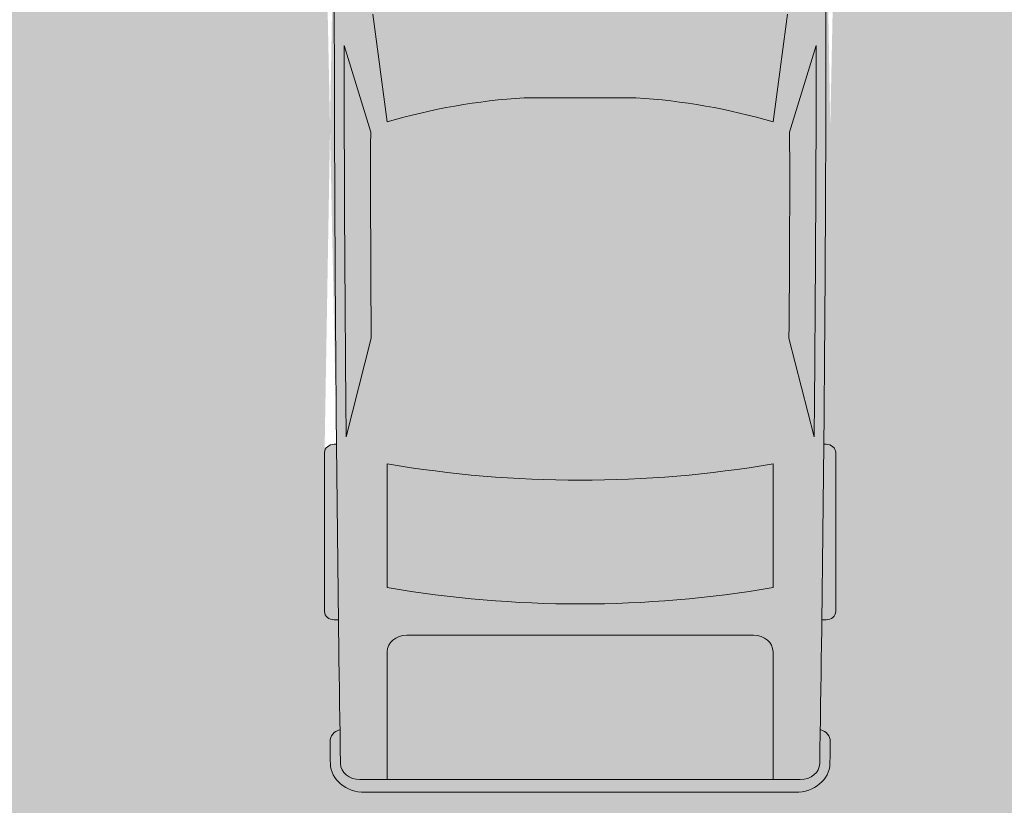
# Model space of a CAD drawing. Units: inches. Extents: x 389 to 971, y 148 to 870.
# Tile 1 of 14: x 448 to 565, y 256 to 349. Entities that reach past the tile are written whole.
import ezdxf

# ---------------------------------------------------------------- set-up
doc = ezdxf.new("R2010")
doc.units = ezdxf.units.IN
doc.header["$MEASUREMENT"] = 0
doc.layers.add('C-VEHI', color=8, linetype='Continuous', lineweight=13)
doc.layers.add('L-GRND-BASE-PATT', color=8, linetype='Continuous', lineweight=13)
doc.layers.add('C-VEHI-PATT', color=18, linetype='Continuous', lineweight=13, true_color=0x000000)
doc.layers.add('L-GRND-PATT', color=39, linetype='Continuous', lineweight=13, true_color=0x603913)

# ---------------------------------------------------------------- blocks, each defined once
blk = doc.blocks.new('*U7')
for p, q in [((136.6978032355602, 38.88847654282876), (160.90094244002, 38.88847654282867)), ((135.4513231603356, 37.07354110333037), (135.4513231603356, 37.40863046792069)), ((162.1474225152445, 37.40863046792049), (162.1474225152445, 36.77402019194128)), ((87.98532186932616, 31.87120872459877), (74.75900729854769, 35.92175679182955)), ((134.313356548143, 35.6043097713567), (119.2882629232503, 31.77757799177584)), ((186.4728846989705, -33.49860931502491), (186.4728846989718, 33.49860931502465)), ((70.0302824853563, 31.53613089391356), (86.40615155322342, 29.35124891408057)), ((188.3990091454065, -32.75868627757393), (188.3990091454077, 32.75868627757058)), ((138.4228833961707, 29.35124891408074), (157.2465674415997, 29.35124891408074)), ((186.4728846989718, 29.35124891408083), (167.0083537481071, 29.35124891408083)), ((164.515393597658, 26.39155676426461), (164.5153935976578, -26.39155676426503)), ((186.4728846989718, -10.5288681329018), (186.4728846989718, 10.52886813290129)), ((82.73706193978568, 8.496039918672748), (82.73706193978568, -8.49603991867258)), ((86.40615155322318, -29.35124891408145), (70.03028248535594, -31.53613089391442)), ((157.2465674415997, -29.35124891408117), (138.4228833961707, -29.35124891408126)), ((167.008353748107, -29.35124891408126), (186.4728846989707, -29.35124891408108)), ((87.98532186932607, -31.87120872459903), (74.7590072985476, -35.92175679182964)), ((134.3133565481428, -35.60430977135721), (119.2882629232503, -31.77757799177618)), ((135.4513231603355, -37.07354110333088), (135.4513231603355, -37.4086304679212)), ((162.1474225152445, -37.408630467921), (162.1474225152445, -36.77402019194179)), ((136.6978032355602, -38.88847654282927), (160.9009424400199, -38.88847654282918))]:
    blk.add_line(p, q)
for centre, major_axis, ratio, start_param, end_param in [((64.48199294511879, -10555.61767587835), (1.907644e-10, 10593.02630634627), 0.842303869543847, -0.0133969486112073, 0.0027970409639888), ((136.6978032355602, 37.40863046792072), (2.357e-13, -1.479846074908118), 0.842303869543976, 3.141592653589603, 4.712388980384554), ((160.90094244002, 37.40863046792052), (5.59e-14, 1.479846074908118), 0.842303869543976, -1.570796326794865, 4.44e-14), ((180.6280394947615, 35.8381667808375), (7.4e-14, 2.219769112362114), 0.8423038695439693, -0.0130174256259048, 1.249894140392862), ((64.48199294754608, -10556.35759891604), (1.349839377e-06, 10595.3130398087), 0.8423038681351469, -0.0133969484821159, -0.0130174254969711), ((183.9799245485216, 32.75868627756583), (8.56e-14, -5.246425615115243), 0.8423038695439737, 1.570796326795794, 3.128195704978164), ((183.9799245485226, 33.49860931502124), (3e-16, -2.959692149816168), 0.8423038695439952, 1.570796326796048, 3.128195704978389), ((64.4819929449925, -10555.61767590795), (1.9177683e-09, -10591.54646030096), 0.8423038695482963, 3.133765086725325, 3.140440689641252), ((95.78879860270445, -3666.353346297651), (1.949864e-10, -3698.236159209632), 0.8423038695446962, 3.134048706297306, 3.14409775411291), ((149.595361812917, 2.799442537139299), (8.561e-13, -79.57966406425402), 0.842303869543983, 4.372215489277867, 4.640744122441986), ((17.08207736189386, -1.421e-13), (6.87e-14, 147.0179238898305), 0.8423038695439764, 4.511394369635731, 4.913383591133647), ((35.90576140732288, -1.421e-13), (6.87e-14, 147.0179238898305), 0.8423038695439764, 4.511394369635731, 4.913383591133647), ((167.0083537481071, 26.39155676426464), (1.394e-13, 2.959692149816236), 0.842303869543976, 5.55e-14, 1.57079632679492), ((149.5953618129329, -2.799442537137565), (4.0897e-12, -79.57966406427697), 0.8423038695439419, -1.499151468852248, -1.230622835688196), ((167.008353748107, -26.39155676426503), (1.02e-14, -2.959692149816192), 0.8423038695439885, 4.712388980384686, 6.283185307179581), ((95.78879860271888, 3666.35334629765), (1.637818e-10, -3698.236159209629), 0.8423038695447546, -0.0025051005232382, 0.007543947292366), ((183.9799245485177, -32.7586862775633), (2.428e-13, -5.246425615118353), 0.8423038695439808, 0.0133969486110846, 1.570796326792831), ((183.9799245485216, -33.4986093150211), (9.3e-15, 2.959692149816141), 0.8423038695439732, 3.154989602201626, 4.71238898038339), ((64.48199294503607, 10555.61767590793), (1.6049794e-09, -10591.54646030094), 0.8423038695397146, 0.0011519639481523, 0.0078275668641468), ((64.48199294495228, 10555.61767590795), (6.117947e-10, 10593.02630637587), 0.8423038695458146, 3.138795612625926, 3.154989602201039), ((136.6978032355602, -37.40863046792109), (1.56e-14, -1.479846074908162), 0.8423038695440105, -1.570796326794875, -1.27e-14), ((160.9009424400199, -37.408630467921), (1.969e-13, 1.479846074908162), 0.8423038695440109, 3.141592653589951, 4.712388980384771), ((180.6280394947581, -35.83816678083949), (2.274e-13, -2.219769112363032), 0.8423038695439803, -1.249894138785958, 0.0130174256254374), ((64.48199294197605, 10556.3575989598), (9.365289701e-07, 10595.31303985772), 0.8423038705260315, 3.154610079306566, 3.154989602290631)]:
    blk.add_ellipse(centre, major_axis=major_axis, ratio=ratio, start_param=start_param, end_param=end_param)

msp = doc.modelspace()

# ---------------------------------------------------------------- hatches: boundary and pattern name
at = {"layer": 'C-VEHI-PATT'}
h = msp.add_hatch(color=256, dxfattribs=at)
h.dxf.hatch_style = 1
edge = h.paths.add_edge_path(flags=16)
edge.add_ellipse((3386.011413077446, 329.726312794031), major_axis=(-2896.629999631248, 1.069454e-10), ratio=0.8423038695494893, start_angle=-0.1208973690315247, end_angle=0.3640763488915013, ccw=False)
edge.add_line((489.3905023836935, 335.8383575186984), (486.2179253655185, 346.1978202249628))
edge.add_ellipse((8782.002602781096, 354.247254279773), major_axis=(-8295.790181758603, 9.87839e-10), ratio=0.8423038695486498, start_angle=0.0555943135052214, end_angle=0.3777641939157137)
edge.add_line((486.4665645878948, 299.5520931219791), (489.4638383140943, 311.3204429697198))
edge = h.paths.add_edge_path(flags=16)
edge.add_ellipse((512.1608573463288, 287.5825181681774), major_axis=(62.33048198263887, 2.0798e-12), ratio=0.8423038695439498, start_angle=94.8700695971331, end_angle=112.791914877584)
edge.add_line((491.3642517254777, 337.0752369161335), (489.6529508739416, 349.9015767089268))
edge.add_ellipse((510.1338164488795, 298.7862183048575), major_axis=(64.04807894948699, 3.9006e-12), ratio=0.8423038695439252, start_angle=94.27742096304979, end_angle=111.83495379670401, ccw=False)
edge.add_line((506.1068129054811, 352.6274231954524), (522.600208125781, 352.6274231954521))
edge.add_ellipse((518.5732045823798, 298.7862183048586), major_axis=(64.04807894948067, 3.24e-14), ratio=0.8423038695439885, start_angle=68.16504620328948, end_angle=85.72257903694378, ccw=False)
edge.add_line((539.05407015732, 349.9015767089259), (537.3427693057835, 337.0752369161327))
edge.add_ellipse((516.5461636849332, 287.5825181681899), major_axis=(62.33048198262021, 1.5954e-12), ratio=0.8423038695439995, start_angle=67.20808512240782, end_angle=85.12993040286212)
edge.add_line((521.0080028322477, 339.9490379899644), (507.6990181990146, 339.9490379899646))
edge = h.paths.add_edge_path(flags=16)
edge.add_ellipse((514.3535105156315, 391.3730654902235), major_axis=(-115.1512533244504, 1.8736e-12), ratio=0.8423038695439684, start_angle=76.4018653097696, end_angle=103.5981346902308)
edge.add_line((537.3427693057832, 296.3333211885938), (537.342769305783, 281.5897392316151))
edge.add_ellipse((514.3535105156313, 376.6294835332447), major_axis=(-115.1512533244486, 9.02e-13), ratio=0.8423038695439828, start_angle=76.40186530976922, end_angle=103.59813469023032, ccw=False)
edge.add_line((491.3642517254773, 281.5897392316156), (491.3642517254774, 296.3333211885945))
edge = h.paths.add_edge_path()
edge.add_ellipse((8782.002602781105, 354.2472542798386), major_axis=(-8296.949265805946, 5.39345e-11), ratio=0.8423038695428886, start_angle=0.3838667787920247, end_angle=0.5282714718170651)
edge.add_ellipse((8782.002602781105, 354.2472542798386), major_axis=(-8296.949265805946, 5.39345e-11), ratio=0.8423038695428886, start_angle=0.5282714718170651, end_angle=0.6465540970606384)
edge.add_ellipse((488.1158467995968, 260.6509346628684), major_axis=(2.318168094668909, 7.48e-14), ratio=0.8423038695439647, start_angle=180.6465540970884, end_angle=269.9999999999081)
edge.add_line((488.115846799593, 258.6983327064755), (491.3642517254771, 258.6983327064753))
edge.add_line((491.3642517254771, 258.6983327064753), (491.3642517254771, 274.201106836649))
edge.add_ellipse((493.6824198201462, 273.9438556676354), major_axis=(-2.318168094668919, 1.896e-13), ratio=0.8423038695439611, start_angle=-89.99999999999523, end_angle=4.718003765447065e-12, ccw=False)
edge.add_line((493.6824198201462, 275.8964576240284), (535.3300149439905, 275.8964576240277))
edge.add_ellipse((535.024601211114, 273.9438556676347), major_axis=(2.318168094668976, 2.946e-13), ratio=0.8423038695439647, start_angle=-7.275957614183426e-12, end_angle=89.99999999998943, ccw=False)
edge.add_line((537.342769305783, 273.9438556676347), (537.3427693057827, 258.698332706474))
edge.add_line((537.3427693057827, 258.698332706474), (540.591174231666, 258.6983327064739))
edge.add_ellipse((540.5911742316634, 260.6509346628669), major_axis=(-2.318168094668839, 2.143e-13), ratio=0.8423038695440144, start_angle=90.00000000008203, end_angle=179.3534459029346)
edge.add_ellipse((-7753.295581726658, 354.2472542799028), major_axis=(-8296.949265782761, 2.068448e-10), ratio=0.8423038695442414, start_angle=179.3534459029388, end_angle=179.3813568036815)
edge.add_ellipse((-7753.295581726658, 354.2472542799028), major_axis=(-8296.949265782761, 2.068448e-10), ratio=0.8423038695442414, start_angle=179.3813568036815, end_angle=179.4717285281828)
edge.add_ellipse((-7753.295581726658, 354.2472542799028), major_axis=(-8296.949265782761, 2.068448e-10), ratio=0.8423038695442414, start_angle=179.4717285281828, end_angle=179.6161332212082)
edge.add_ellipse((-7753.295581726658, 354.2472542799028), major_axis=(-8296.949265782761, 2.068448e-10), ratio=0.8423038695442414, start_angle=179.6161332212082, end_angle=180.090229088595)
edge.add_ellipse((-7753.295581726658, 354.2472542799028), major_axis=(-8296.949265782761, 2.068448e-10), ratio=0.8423038695442414, start_angle=180.090229088595, end_angle=180.134986576859)
edge.add_ellipse((129.8867725257751, 372.4897205359271), major_axis=(-413.7373561031673, 2.44623e-11), ratio=0.8423038695441432, start_angle=180.1806905311865, end_angle=182.1799503136479)
edge.add_ellipse((129.8867725257751, 372.4897205359271), major_axis=(-413.7373561031673, 2.44623e-11), ratio=0.8423038695441432, start_angle=182.1799503136479, end_angle=183.6504275857017)
edge.add_ellipse((492.7951034259847, 196.3854951855023), major_axis=(245.3971626940514, 1.422861e-10), ratio=0.8423038695444116, start_angle=76.21947101046817, end_angle=77.87403444768196)
edge.add_ellipse((49.13479434038987, 375.4013592680261), major_axis=(-488.2195497741754, 2.5232e-12), ratio=0.8423038695439587, start_angle=177.8014594340445, end_angle=182.8637146078372, ccw=False)
edge.add_ellipse((518.5732045823792, 299.4839331720493), major_axis=(-70.31786407385354, 1.4408e-12), ratio=0.8423038695439844, start_angle=252.2800467772501, end_angle=265.9175893088498)
edge.add_line((522.79289864913, 358.606202334111), (505.9141223821329, 358.6062023341113))
edge.add_ellipse((510.1338164488812, 299.4839331720496), major_axis=(70.3178640738586, 3.814e-12), ratio=0.8423038695439212, start_angle=94.08241069114636, end_angle=107.7199532227462)
edge.add_ellipse((979.5722266908713, 375.4013592680145), major_axis=(-488.2195497741742, 7.7268e-12), ratio=0.842303869543895, start_angle=-2.863714607837494, end_angle=2.198540565955284, ccw=False)
edge.add_ellipse((535.9119176052733, 196.3854951855018), major_axis=(-245.3971626940985, 1.013648e-10), ratio=0.8423038695442548, start_angle=-77.87403444769295, end_angle=-76.2194710104792)
edge.add_ellipse((898.8202485054873, 372.489720535918), major_axis=(413.7373561031672, 1.26113e-11), ratio=0.8423038695441164, start_angle=176.3495724142985, end_angle=177.8200496863523)
edge.add_ellipse((898.8202485054873, 372.489720535918), major_axis=(413.7373561031672, 1.26113e-11), ratio=0.8423038695441164, start_angle=177.8200496863523, end_angle=179.8643876095591)
edge.add_ellipse((8782.002602781105, 354.2472542798386), major_axis=(-8296.949265805946, 5.39345e-11), ratio=0.8423038695428886, start_angle=-0.1349865768573029, end_angle=-0.090229088593484)
edge.add_ellipse((8782.002602781105, 354.2472542798386), major_axis=(-8296.949265805946, 5.39345e-11), ratio=0.8423038695428886, start_angle=-0.090229088593484, end_angle=0.3838667787920247)
edge = h.paths.add_edge_path(flags=16)
edge.add_ellipse((-2357.304392046186, 329.7263127941099), major_axis=(2896.629999631251, 5.35614e-11), ratio=0.8423038695445265, start_angle=-0.3640763488920631, end_angle=0.1208973690309369)
edge.add_line((539.3165186475693, 335.8383575187012), (542.4890956657468, 346.1978202249727))
edge.add_ellipse((-7753.295581749842, 354.2472542800017), major_axis=(8295.790181758617, 3.2664368e-09), ratio=0.8423038695525207, start_angle=-0.37776419393310334, end_angle=-0.055594313522590255, ccw=False)
edge.add_line((542.240456443367, 299.5520931219743), (539.2431827171666, 311.3204429697195))
h = msp.add_hatch(color=256, dxfattribs=at)
h.dxf.hatch_style = 1
edge = h.paths.add_edge_path()
edge.add_ellipse((518.5732045823798, 298.7862183048586), major_axis=(64.04807894948067, 3.24e-14), ratio=0.8423038695439885, start_angle=68.16504620328955, end_angle=85.72257903694374)
edge.add_line((522.600208125781, 352.6274231954521), (506.106812905481, 352.6274231954524))
edge.add_ellipse((510.1338164488795, 298.7862183048575), major_axis=(64.04807894948699, 3.9006e-12), ratio=0.8423038695439252, start_angle=94.2774209630498, end_angle=111.834953796704)
edge.add_line((489.6529508739416, 349.9015767089268), (491.3642517254777, 337.0752369161335))
edge.add_ellipse((512.1608573463288, 287.5825181681774), major_axis=(62.33048198263887, 2.0798e-12), ratio=0.8423038695439498, start_angle=94.87006959713312, end_angle=112.79191487758399, ccw=False)
edge.add_line((507.6990181990146, 339.9490379899646), (521.0080028322477, 339.9490379899644))
edge.add_ellipse((516.5461636849332, 287.5825181681899), major_axis=(62.33048198262021, 1.5954e-12), ratio=0.8423038695439995, start_angle=67.2080851224078, end_angle=85.1299304028621, ccw=False)
edge.add_line((537.3427693057835, 337.0752369161327), (539.05407015732, 349.9015767089259))
h = msp.add_hatch(color=256, dxfattribs=at)
h.dxf.hatch_style = 1
edge = h.paths.add_edge_path()
edge.add_ellipse((3386.011413077446, 329.726312794031), major_axis=(-2896.629999631248, 1.069454e-10), ratio=0.8423038695494893, start_angle=-0.1208973690315247, end_angle=0.3640763488915013, ccw=False)
edge.add_line((489.3905023836935, 335.8383575186984), (486.2179253655185, 346.1978202249628))
edge.add_ellipse((8782.002602781096, 354.247254279773), major_axis=(-8295.790181758603, 9.87839e-10), ratio=0.8423038695486498, start_angle=0.0555943135052214, end_angle=0.3777641939157137)
edge.add_line((486.4665645878948, 299.5520931219791), (489.4638383140943, 311.3204429697198))
h = msp.add_hatch(color=256, dxfattribs=at)
h.dxf.hatch_style = 1
edge = h.paths.add_edge_path()
edge.add_ellipse((-7753.295581749842, 354.2472542800017), major_axis=(8295.790181758617, 3.2664368e-09), ratio=0.8423038695525207, start_angle=-0.3777641939330845, end_angle=-0.0555943135225903)
edge.add_line((542.4890956657468, 346.1978202249726), (539.3165186475693, 335.8383575187011))
edge.add_ellipse((-2357.304392046186, 329.7263127941099), major_axis=(2896.629999631251, 5.35614e-11), ratio=0.8423038695445265, start_angle=-0.3640763488921266, end_angle=0.12089736903089943, ccw=False)
edge.add_line((539.2431827171666, 311.3204429697195), (542.240456443367, 299.5520931219743))
h = msp.add_hatch(color=256, dxfattribs=at)
h.dxf.hatch_style = 1
edge = h.paths.add_edge_path()
edge.add_line((519.1534714069603, 339.9490379899644), (509.5535496243029, 339.9490379899646))
edge.add_line((509.5535496243029, 339.9490379899646), (509.5535496243029, 294.4650205384671))
edge.add_ellipse((514.3535105156315, 391.3730654902235), major_axis=(-115.1512533244504, 1.8736e-12), ratio=0.8423038695439684, start_angle=87.16439508461924, end_angle=92.83560491538267)
edge.add_line((519.1534714069603, 294.4650205384671), (519.1534714069603, 339.9490379899644))
h = msp.add_hatch(color=256, dxfattribs=at)
h.dxf.hatch_style = 1
edge = h.paths.add_edge_path()
edge.add_ellipse((8782.002602781105, 354.2472542798386), major_axis=(-8296.949265805946, 5.39345e-11), ratio=0.8423038695428886, start_angle=0.3838667787920258, end_angle=0.5282714718171064, ccw=False)
edge.add_line((485.3157944992978, 298.6607849184044), (485.0533369751561, 298.6607849184044))
edge.add_ellipse((485.053336975156, 297.6844839402078), major_axis=(1.159084047334488, 1.025e-13), ratio=0.8423038695440382, start_angle=89.99999999999493, end_angle=179.9999999999949)
edge.add_line((483.8942529278216, 297.6844839402078), (483.8942529278214, 278.7274633263938))
edge.add_ellipse((485.0533369751559, 278.7274633263938), major_axis=(-1.159084047334545, 3.11e-13), ratio=0.8423038695439968, start_angle=1.53667e-11, end_angle=90.000000000012)
edge.add_line((485.0533369751558, 277.7511623481972), (485.5503931620382, 277.7511623481972))
h = msp.add_hatch(color=256, dxfattribs=at)
h.dxf.hatch_style = 1
edge = h.paths.add_edge_path()
edge.add_ellipse((543.6536840561046, 297.6844839402071), major_axis=(1.159084047334431, 1.769e-13), ratio=0.8423038695439814, start_angle=-1.15625e-11, end_angle=89.99999999999125)
edge.add_line((543.6536840561046, 298.6607849184036), (543.3912265319653, 298.6607849184036))
edge.add_ellipse((-7753.295581726658, 354.2472542799028), major_axis=(-8296.949265782761, 2.068448e-10), ratio=0.8423038695442414, start_angle=179.4717285281829, end_angle=179.6161332212083, ccw=False)
edge.add_line((543.1566278692261, 277.7511623481965), (543.6536840561052, 277.7511623481965))
edge.add_ellipse((543.6536840561043, 278.727463326393), major_axis=(-1.159084047334431, 2.574e-13), ratio=0.8423038695440306, start_angle=90.0000000000127, end_angle=180.0000000000099)
edge.add_line((544.8127681034387, 278.7274633263929), (544.8127681034391, 297.684483940207))
h = msp.add_hatch(color=256, dxfattribs=at)
h.dxf.hatch_style = 1
edge = h.paths.add_edge_path()
edge.add_ellipse((514.3535105156315, 391.3730654902235), major_axis=(-115.1512533244504, 1.8736e-12), ratio=0.8423038695439684, start_angle=76.40186530976962, end_angle=103.59813469023078, ccw=False)
edge.add_line((491.3642517254774, 296.3333211885945), (491.3642517254773, 281.5897392316156))
edge.add_ellipse((514.3535105156313, 376.6294835332447), major_axis=(-115.1512533244486, 9.02e-13), ratio=0.8423038695439828, start_angle=76.40186530976916, end_angle=103.5981346902303)
edge.add_line((537.342769305783, 281.5897392316151), (537.3427693057832, 296.3333211885938))
h = msp.add_hatch(color=256, dxfattribs=at)
h.dxf.hatch_style = 1
edge = h.paths.add_edge_path()
edge.add_ellipse((540.0116322079951, 260.6509346628677), major_axis=(-4.109243751168186, 2.384e-13), ratio=0.842303869543976, start_angle=90.0000000000635, end_angle=179.3534459029232)
edge.add_ellipse((-7753.875123750511, 354.2472542780016), major_axis=(-8298.740341433751, 2.4782644722e-06), ratio=0.8423038662721074, start_angle=179.3534459200609, end_angle=179.371762800894)
edge.add_ellipse((542.4236240941387, 263.2762864208561), major_axis=(-1.738626071001761, 2.132e-13), ratio=0.8423038695439151, start_angle=179.3717627838137, end_angle=248.464756601011)
edge.add_ellipse((-7753.295581726658, 354.2472542799028), major_axis=(-8296.949265782761, 2.068448e-10), ratio=0.8423038695442414, start_angle=179.3534459029389, end_angle=179.3813568036816, ccw=False)
edge.add_ellipse((540.5911742316634, 260.6509346628669), major_axis=(-2.318168094668839, 2.143e-13), ratio=0.8423038695440144, start_angle=90.00000000008203, end_angle=179.3534459029347, ccw=False)
edge.add_line((540.5911742316662, 258.6983327064739), (488.1158467995929, 258.6983327064755))
edge.add_ellipse((488.1158467995968, 260.6509346628684), major_axis=(2.318168094668909, 7.48e-14), ratio=0.8423038695439647, start_angle=180.6465540970884, end_angle=269.99999999990814, ccw=False)
edge.add_ellipse((8782.002602781105, 354.2472542798386), major_axis=(-8296.949265805946, 5.39345e-11), ratio=0.8423038695428886, start_angle=0.5282714718171064, end_angle=0.6465540970606867, ccw=False)
edge.add_ellipse((486.2833969371199, 263.2762864208594), major_axis=(-1.738626071002378, 2.7e-13), ratio=0.8423038695439394, start_angle=-68.4647564959682, end_angle=0.6282372161795267)
edge.add_ellipse((8782.582144816053, 354.2472542821698), major_axis=(-8298.740341477976, 1.8591886369e-06), ratio=0.8423038720186145, start_angle=0.6282372290785363, end_angle=0.6465541099115812)
edge.add_ellipse((488.6953888232669, 260.6509346628715), major_axis=(4.10924375117072, 1.262e-13), ratio=0.8423038695439824, start_angle=180.6465540970564, end_angle=269.9999999998589)
edge.add_line((488.6953888232593, 257.1897027503609), (540.0116322079989, 257.1897027503593))
h = msp.add_hatch(color=256, dxfattribs=at)
h.dxf.hatch_style = 1
edge = h.paths.add_edge_path()
edge.add_ellipse((514.3535105156313, 376.6294835332447), major_axis=(-115.1512533244486, 9.02e-13), ratio=0.8423038695439828, start_angle=87.16439508461889, end_angle=92.83560491538242, ccw=False)
edge.add_line((509.5535496243029, 279.7214385814882), (509.5535496243029, 275.8964576240281))
edge.add_line((509.5535496243029, 275.8964576240281), (519.1534714069603, 275.896457624028))
edge.add_line((519.1534714069603, 275.896457624028), (519.1534714069603, 279.7214385814881))
h = msp.add_hatch(color=256, dxfattribs=at)
h.dxf.hatch_style = 1
edge = h.paths.add_edge_path()
edge.add_ellipse((535.024601211114, 273.9438556676347), major_axis=(2.318168094668976, 2.946e-13), ratio=0.8423038695439647, start_angle=-7.2761e-12, end_angle=89.99999999998938)
edge.add_line((535.0246012111141, 275.8964576240277), (493.6824198201462, 275.8964576240284))
edge.add_ellipse((493.6824198201462, 273.9438556676354), major_axis=(-2.318168094668919, 1.896e-13), ratio=0.8423038695439611, start_angle=-89.99999999999532, end_angle=4.6829e-12)
edge.add_line((491.3642517254771, 273.9438556676347), (491.3642517254771, 258.6983327064753))
edge.add_line((491.3642517254771, 258.6983327064753), (537.3427693057827, 258.698332706474))
edge.add_line((537.3427693057827, 258.698332706474), (537.342769305783, 273.9438556676347))
at = {"layer": 'L-GRND-BASE-PATT'}
h = msp.add_hatch(color=256, dxfattribs=at)
h.dxf.hatch_style = 1
edge = h.paths.add_edge_path(flags=16)
edge.add_ellipse((8782.002602781105, 354.2472542798386), major_axis=(-8296.949265805946, 5.39345e-11), ratio=0.8423038695428886, start_angle=-0.0902290885933894, end_angle=0.3838667787920258, ccw=False)
edge.add_ellipse((485.0533369751568, 368.2895347624687), major_axis=(-1.159084047334488, 1.838e-13), ratio=0.8423038695439892, start_angle=9.094947017729282e-12, end_angle=90.00000000000898, ccw=False)
edge.add_line((483.8942529278224, 368.2895347624687), (483.8942529278225, 387.6039063360424))
edge.add_ellipse((485.0533369751571, 387.2465553762829), major_axis=(1.159084047334488, 1.838e-13), ratio=0.8423038695439892, start_angle=89.99999999999102, end_angle=179.9999999999909, ccw=False)
edge.add_line((485.0533369751572, 388.2228563544795), (485.5047440247956, 388.2228563544795))
edge.add_ellipse((898.8202485054873, 372.489720535918), major_axis=(413.7373561031672, 1.26113e-11), ratio=0.8423038695441164, start_angle=176.3495724142986, end_angle=177.8200496863524, ccw=False)
edge.add_ellipse((535.9119176052733, 196.3854951855018), major_axis=(-245.3971626940985, 1.013648e-10), ratio=0.8423038695442548, start_angle=-77.87403444769302, end_angle=-76.2194710104792, ccw=False)
edge.add_ellipse((535.9119176052684, 201.7546502845751), major_axis=(239.1273775699096, 1.008988e-10), ratio=0.842303869543627, start_angle=100.20953899711827, end_angle=102.44462729341922, ccw=False)
edge.add_ellipse((473.3138688667988, 564.9222417143382), major_axis=(196.5636751472093, 8.4793e-12), ratio=0.8423038695439335, start_angle=-80.74343399280163, end_angle=-77.44506735586587)
edge.add_line((509.5535496243029, 402.1940957519602), (514.3535105156315, 404.8483349684994))
edge.add_line((514.3535105156315, 404.8483349684994), (514.3535105156315, 404.7971763262221))
edge.add_ellipse((514.3535105156316, 404.2643898676136), major_axis=(0.5795420236673633, 2e-16), ratio=0.8423038695437671, start_angle=52.06686954015339, end_angle=90.00000000001342, ccw=False)
edge.add_line((514.671564037824, 404.672460591463), (519.1534714069603, 402.19409575196))
edge.add_ellipse((555.3931521644682, 564.9222417143374), major_axis=(-196.5636751472384, 3.62381e-11), ratio=0.8423038695438114, start_angle=77.44506735587258, end_angle=80.74343399280833)
edge.add_ellipse((492.795103425985, 201.7546502845724), major_axis=(239.12737756976, 4.82267e-11), ratio=0.8423038695441539, start_angle=77.55537270654253, end_angle=79.7904610028433, ccw=False)
edge.add_ellipse((492.7951034259847, 196.3854951855023), major_axis=(245.3971626940514, 1.422861e-10), ratio=0.8423038695444116, start_angle=76.21947101046823, end_angle=77.87403444768199, ccw=False)
edge.add_ellipse((129.8867725257751, 372.4897205359271), major_axis=(-413.7373561031673, 2.44623e-11), ratio=0.8423038695441432, start_angle=182.179950313648, end_angle=183.6504275857018, ccw=False)
edge.add_line((543.2022770064673, 388.2228563544788), (544.0779382625514, 388.2228563544787))
edge.add_ellipse((543.6536840561057, 387.2465553762822), major_axis=(-1.159084047334545, 1.527e-13), ratio=0.8423038695438989, start_angle=180.0000000000075, end_angle=270.00000000000756, ccw=False)
edge.add_line((544.8127681034401, 387.2465553762826), (544.8127681034399, 367.9321838027083))
edge.add_ellipse((543.6536840561054, 368.2895347624679), major_axis=(1.159084047334544, 7.24e-14), ratio=0.8423038695439478, start_angle=269.9999999999964, end_angle=359.9999999999964, ccw=False)
edge.add_ellipse((-7753.295581726658, 354.2472542799028), major_axis=(-8296.949265782761, 2.068448e-10), ratio=0.8423038695442414, start_angle=179.6161332212083, end_angle=180.0902290885951, ccw=False)
edge.add_line((543.3912265319653, 298.6607849184036), (544.0779382625504, 298.6607849184036))
edge.add_ellipse((543.6536840561046, 297.6844839402071), major_axis=(1.159084047334431, 1.769e-13), ratio=0.8423038695439814, start_angle=-1.1482370609883219e-11, end_angle=89.99999999999119, ccw=False)
edge.add_line((544.8127681034391, 297.684483940207), (544.8127681034387, 278.3701123666333))
edge.add_ellipse((543.6536840561043, 278.727463326393), major_axis=(-1.159084047334431, 2.574e-13), ratio=0.8423038695440306, start_angle=90.00000000001268, end_angle=180.0000000000099, ccw=False)
edge.add_line((543.6536840561045, 277.7511623481965), (543.1566278692261, 277.7511623481965))
edge.add_ellipse((-7753.295581726658, 354.2472542799028), major_axis=(-8296.949265782761, 2.068448e-10), ratio=0.8423038695442414, start_angle=179.3813568036816, end_angle=179.4717285281829, ccw=False)
edge.add_ellipse((542.4236240941387, 263.2762864208561), major_axis=(-1.738626071001761, 2.132e-13), ratio=0.8423038695439151, start_angle=179.3717627838137, end_angle=248.464756601011, ccw=False)
edge.add_ellipse((-7753.875123750511, 354.2472542780016), major_axis=(-8298.740341433751, 2.4782644722e-06), ratio=0.8423038662721074, start_angle=179.3534459200609, end_angle=179.3717628008941, ccw=False)
edge.add_ellipse((540.0116322079951, 260.6509346628677), major_axis=(-4.109243751168186, 2.384e-13), ratio=0.842303869543976, start_angle=90.0000000000635, end_angle=179.3534459029233, ccw=False)
edge.add_line((540.0116322079991, 257.1897027503593), (488.6953888232593, 257.1897027503609))
edge.add_ellipse((488.6953888232669, 260.6509346628715), major_axis=(4.10924375117072, 1.262e-13), ratio=0.8423038695439824, start_angle=180.6465540970565, end_angle=269.9999999998589, ccw=False)
edge.add_ellipse((8782.582144816053, 354.2472542821698), major_axis=(-8298.740341477976, 1.8591886369e-06), ratio=0.8423038720186145, start_angle=0.6282372290784792, end_angle=0.6465541099116194, ccw=False)
edge.add_ellipse((486.2833969371199, 263.2762864208594), major_axis=(-1.738626071002378, 2.7e-13), ratio=0.8423038695439394, start_angle=-68.46475649596817, end_angle=0.6282372161796275, ccw=False)
edge.add_ellipse((8782.002602781105, 354.2472542798386), major_axis=(-8296.949265805946, 5.39345e-11), ratio=0.8423038695428886, start_angle=0.5282714718171064, end_angle=0.6465540970606867, ccw=False)
edge.add_line((485.5503931620382, 277.7511623481972), (484.6290827687102, 277.7511623481972))
edge.add_ellipse((485.0533369751559, 278.7274633263938), major_axis=(-1.159084047334545, 3.11e-13), ratio=0.8423038695439968, start_angle=1.5404566511278972e-11, end_angle=90.000000000012, ccw=False)
edge.add_line((483.8942529278214, 278.7274633263938), (483.8942529278216, 298.0418348999672))
edge.add_ellipse((485.053336975156, 297.6844839402078), major_axis=(1.159084047334488, 1.025e-13), ratio=0.8423038695440382, start_angle=89.99999999999488, end_angle=179.9999999999949, ccw=False)
edge = h.paths.add_edge_path(flags=0)
edge.add_ellipse((8782.002602781096, 354.247254279773), major_axis=(-8295.790181758603, 9.87839e-10), ratio=0.8423038695486498, start_angle=0.05559431350519617, end_angle=0.37776419391582294, ccw=False)
edge.add_line((486.2179253655185, 346.1978202249628), (489.3905023836935, 335.8383575186984))
edge.add_ellipse((3386.011413077446, 329.726312794031), major_axis=(-2896.629999631248, 1.069454e-10), ratio=0.8423038695494893, start_angle=-0.1208973690315206, end_angle=0.3640763488915184)
edge.add_line((489.4638383140943, 311.3204429697198), (486.4665645878948, 299.5520931219791))
edge = h.paths.add_edge_path(flags=0)
edge.add_ellipse((514.3535105156315, 391.3730654902235), major_axis=(-115.1512533244504, 1.8736e-12), ratio=0.8423038695439684, start_angle=76.4018653097696, end_angle=103.5981346902308)
edge.add_line((537.3427693057832, 296.3333211885938), (537.342769305783, 281.5897392316151))
edge.add_ellipse((514.3535105156313, 376.6294835332447), major_axis=(-115.1512533244486, 9.02e-13), ratio=0.8423038695439828, start_angle=76.40186530976922, end_angle=103.59813469023032, ccw=False)
edge.add_line((491.3642517254773, 281.5897392316156), (491.3642517254774, 296.3333211885945))
edge = h.paths.add_edge_path(flags=0)
edge.add_line((491.3642517254777, 337.0752369161334), (489.6529508739416, 349.9015767089268))
edge.add_ellipse((510.1338164488795, 298.7862183048575), major_axis=(64.04807894948699, 3.9006e-12), ratio=0.8423038695439252, start_angle=94.27742096304979, end_angle=111.83495379670401, ccw=False)
edge.add_line((506.106812905481, 352.6274231954524), (522.600208125781, 352.6274231954521))
edge.add_ellipse((518.5732045823798, 298.7862183048586), major_axis=(64.04807894948067, 3.24e-14), ratio=0.8423038695439885, start_angle=68.16504620328948, end_angle=85.72257903694378, ccw=False)
edge.add_line((539.05407015732, 349.9015767089259), (537.3427693057835, 337.0752369161327))
edge.add_ellipse((516.5461636849332, 287.5825181681899), major_axis=(62.33048198262021, 1.5954e-12), ratio=0.8423038695439995, start_angle=67.20808512240782, end_angle=85.12993040286212)
edge.add_line((521.0080028322477, 339.9490379899644), (507.6990181990146, 339.9490379899646))
edge.add_ellipse((512.1608573463288, 287.5825181681774), major_axis=(62.33048198263887, 2.0798e-12), ratio=0.8423038695439498, start_angle=94.8700695971331, end_angle=112.791914877584)
edge = h.paths.add_edge_path(flags=0)
edge.add_ellipse((493.6824198201462, 273.9438556676354), major_axis=(-2.318168094668919, 1.896e-13), ratio=0.8423038695439611, start_angle=-89.99999999999523, end_angle=4.718003765447065e-12, ccw=False)
edge.add_line((493.6824198201462, 275.8964576240284), (535.3743409680425, 275.8964576240277))
edge.add_ellipse((535.024601211114, 273.9438556676347), major_axis=(2.318168094668976, 2.946e-13), ratio=0.8423038695439647, start_angle=-7.275957614183426e-12, end_angle=89.99999999998943, ccw=False)
edge.add_line((537.342769305783, 273.9438556676347), (537.3427693057827, 258.698332706474))
edge.add_line((537.3427693057827, 258.698332706474), (540.5911742316662, 258.6983327064739))
edge.add_ellipse((540.5911742316634, 260.6509346628669), major_axis=(-2.318168094668839, 2.143e-13), ratio=0.8423038695440144, start_angle=90.00000000008203, end_angle=179.3534459029346)
edge.add_line((540.5911742316662, 258.6983327064739), (487.7691399811528, 258.6983327064755))
edge.add_ellipse((488.1158467995968, 260.6509346628684), major_axis=(2.318168094668909, 7.48e-14), ratio=0.8423038695439647, start_angle=180.6465540970884, end_angle=269.9999999999081)
edge.add_line((488.1158467995931, 258.6983327064755), (491.3642517254771, 258.6983327064754))
edge.add_line((491.3642517254771, 258.6983327064754), (491.3642517254771, 274.2384428182294))
h.paths.add_polyline_path([(746.1375687288224, 327.3223047166553), (750.1400147212453, 327.3223047166553), (750.1400147212453, 326.2830696147227), (798.1693712998389, 326.2830696147227), (798.1693712998389, 327.3223047166553), (802.1718172922616, 327.3223047166553), (802.1718172922616, 309.9783792024682, -0.1904762075443491), (746.1375687288224, 309.9783668090107)], flags=16)
h.paths.add_polyline_path([(782.1595875801748, 313.5684994305933), (782.1595893317732, 309.0414930416419, -0.0496282101666581), (766.1497986905329, 309.0414910503953), (766.1498004421323, 313.5684994305933)], flags=0)
h.paths.add_polyline_path([(755.1858908233534, 344.9352232902417), (755.1858908233534, 373.916311072083), (788.1243995226009, 373.916311072083), (788.1243995226009, 344.9352232902417)], flags=16)
h.paths.add_polyline_path([(757.1858908233535, 346.9352232902417), (757.1858908233535, 371.916311072083), (786.1243995226009, 371.916311072083), (786.1243995226009, 346.9352232902417)], flags=0)
h.paths.add_polyline_path([(803.6445810111745, 338.4878931208803), (803.6445810111745, 342.4903391133031), (804.6838161131072, 342.4903391133031), (804.6838161131072, 390.5196956918968), (803.6445810111748, 390.5196956918968), (803.6445810111748, 394.5221416843196), (820.9885065253617, 394.5221416843196, -0.1904762075443491), (820.9885189188192, 338.4878931208803)], flags=16)
h.paths.add_polyline_path([(806.8706930931005, 326.6963103558256), (806.4254411777042, 327.1415622712219), (806.4723791864895, 326.6297175483474)], flags=16)
h.paths.add_polyline_path([(822.0328146004263, 317.4007976138144), (822.1941503181826, 317.8932883068639), (821.562628166435, 317.9885306563034)], flags=16)
h.paths.add_polyline_path([(817.3983862972365, 358.5001248341902), (817.3983862972365, 374.5099119722327), (821.9253926861879, 374.5099137238312, -0.049628210166658), (821.9253946774346, 358.5001230825909)], flags=0)
h.paths.add_polyline_path([(808.1446344648577, 418.9736619306146), (808.2246858861593, 418.5632188717996), (808.5395491501399, 418.5787472453325)], flags=16)
h.paths.add_polyline_path([(820.3158762739024, 412.6690288868844), (820.4772119916585, 413.161519579934), (819.8456898399113, 413.2567619293735)], flags=16)
h.paths.add_polyline_path([(466.3155093563569, 235.5246322146605), (517.3806533266912, 235.5246322146605), (517.3806533266912, 244.4269231682286), (466.3155093563569, 244.4269231682286)], flags=24)
h.paths.add_polyline_path([(739.8737195480014, 256.2000079819968), (815.4040239338423, 256.2000079819968), (815.4040239338423, 265.3453807094367), (739.8737195480014, 265.3453807094367)], flags=24)
h.paths.add_polyline_path([(750.6081538187397, 393.6666679930368), (791.5680640722773, 393.6666679930368), (791.5680640722773, 412.3933175868746), (750.6081538187397, 412.3933175868746)], flags=24)
h.paths.add_polyline_path([(438.9630812812552, 410.0618566955462), (484.6203810968238, 410.0618566955462), (484.6203810968238, 429.1217352891893), (438.9630812812552, 429.1217352891893)], flags=24)
edge = h.paths.add_edge_path()
edge.add_line((839.2160244416713, 285.6445131961097), (611.8786784019748, 285.6445131961099))
edge.add_line((611.8786784019748, 285.6445131961099), (604.3870116090119, 285.6445131961097))
edge.add_line((604.3870116090119, 285.6445131961097), (595.3870116090119, 285.6445131961097))
edge.add_line((595.3870116090119, 285.6445131961097), (595.3870116090118, 370.1553848722774))
edge.add_line((595.3870116090118, 370.1553848722774), (604.0816928471932, 370.1553848722774))
edge.add_line((604.0816928471932, 370.1553848722774), (604.0816928471932, 371.3788335667469))
edge.add_line((604.0816928471932, 371.3788335667469), (632.0194586761203, 371.3788335667469))
edge.add_arc((604.0816928471932, 370.1553848722773), 27.96454158787471, 2.507490703587644, 90.00000000000003)
edge.add_line((604.0816928471932, 398.1199264601519), (599.8870116090108, 398.1652144688576))
edge.add_line((599.8870116090108, 398.1652144688576), (604.4225424425357, 398.1652144688576))
edge.add_arc((604.4225424425357, 428.4020866923496), 30.23687222349201, 270.0000000000002, 357.492509296413)
edge.add_line((634.6304631740308, 427.0792235325719), (604.4225424425357, 427.0792235325719))
edge.add_line((604.4225424425357, 427.0792235325719), (604.4225424425357, 428.4020866923497))
edge.add_line((604.4225424425357, 428.4020866923497), (599.8870116090119, 428.4020866923497))
edge.add_line((599.8870116090119, 428.4020866923497), (595.3870116090116, 428.4020866923497))
edge.add_line((595.3870116090116, 428.4020866923497), (595.3870116090118, 434.6445131961097))
edge.add_line((595.3870116090118, 434.6445131961097), (585.0790669792458, 434.6445131961097))
edge.add_line((585.0790669792458, 434.6445131961097), (540.3921730610418, 434.6445131961097))
edge.add_line((540.3921730610418, 434.6445131961097), (526.712508448134, 434.6445131961097))
edge.add_line((526.712508448134, 434.6445131961097), (488.4094553949635, 434.6445131961097))
edge.add_line((488.4094553949635, 434.6445131961097), (432.2160244416713, 434.6445131961097))
edge.add_line((432.2160244416713, 434.6445131961097), (432.2160244416713, 243.6445131961098))
edge.add_line((432.2160244416713, 243.6445131961098), (437.2160244416714, 243.6445131961098))
edge.add_line((437.2160244416714, 243.6445131961098), (437.2160244416714, 234.6445131961098))
edge.add_line((437.2160244416714, 234.6445131961098), (581.2160244416713, 234.6445131961098))
edge.add_line((581.2160244416713, 234.6445131961098), (581.2160244416713, 238.6445131961097))
edge.add_line((581.2160244416713, 238.6445131961097), (581.2160244416713, 243.6445131961098))
edge.add_line((581.2160244416713, 243.6445131961098), (590.2160244416713, 243.6445131961098))
edge.add_line((590.2160244416713, 243.6445131961098), (590.2160244416713, 238.6445131961097))
edge.add_line((590.2160244416713, 238.6445131961097), (839.2160244416713, 238.6445131961098))
edge.add_line((839.2160244416713, 238.6445131961098), (839.2160244416713, 285.6445131961097))
at = {"layer": 'L-GRND-PATT'}
h = msp.add_hatch(dxfattribs=at)
h.set_pattern_fill('EARTH', color=256, angle=45)
h.set_pattern_definition([(45, (0, 0), (0, 8.980256121069154), [6.349999999999999, -6.349999999999999]), (45, (-1.683798022700466, 1.683798022700466), (0, 8.980256121069154), [6.349999999999999, -6.349999999999999]), (45, (-3.367596045400933, 3.367596045400933), (0, 8.980256121069154), [6.349999999999999, -6.349999999999999]), (135, (-3.367596045400933, 4.490128060534576), (-8.980256121069154, 0), [6.349999999999999, -6.349999999999999]), (135, (-1.683798022700466, 6.173926083235043), (-8.980256121069154, 0), [6.349999999999999, -6.349999999999999]), (135, (0, 7.85772410593551), (-8.980256121069154, 0), [6.349999999999999, -6.349999999999999])])
h.paths.add_polyline_path([(432.2160244416713, 243.6445131961098), (437.2160244416714, 243.6445131961098), (437.2160244416714, 234.6445131961098), (581.2160244416713, 234.6445131961098), (581.2160244416713, 238.6445131961097), (581.2160244416713, 243.6445131961098), (590.2160244416713, 243.6445131961098), (590.2160244416713, 238.6445131961097), (839.2160244416713, 238.6445131961098), (839.2160244416712, 285.6445131961097), (810.0513609197296, 285.6445131961097), (733.8056934525983, 285.6445131961099), (684.2433676403508, 285.6445131961098), (611.8786784019748, 285.6445131961099), (604.3870116090119, 285.6445131961097), (595.3870116090119, 285.6445131961097), (595.3870116090118, 370.1553848722774), (604.0816928471932, 370.1553848722774), (604.0816928471932, 371.3788335667469), (632.0194586761203, 371.3788335667469, 0.4014527144963568), (604.0816928471932, 398.119926460152), (599.8870116090127, 398.1652144688576), (604.4225424425357, 398.1652144688576, 0.4014527144963579), (634.6304631740308, 427.0792235325719), (604.4225424425357, 427.0792235325719), (604.4225424425357, 428.4020866923497), (599.8870116090119, 428.4020866923497), (595.3870116090116, 428.4020866923497), (595.3870116090118, 434.6445131961097), (585.0790669792458, 434.6445131961097), (540.3921730610418, 434.6445131961097), (526.712508448134, 434.6445131961097), (488.4094553949635, 434.6445131961097), (432.2160244416713, 434.6445131961097)])
edge = h.paths.add_edge_path(flags=16)
edge.add_line((483.8942529278214, 278.7274633263938), (483.8942529278216, 298.2563878122772))
edge.add_ellipse((485.053336975156, 297.6844839402078), major_axis=(1.159084047334488, 1.025e-13), ratio=0.8423038695440382, start_angle=89.99999999999488, end_angle=179.9999999999949, ccw=False)
edge.add_ellipse((8782.002602781105, 354.2472542798386), major_axis=(-8296.949265805946, 5.39345e-11), ratio=0.8423038695428886, start_angle=-0.0902290885933894, end_angle=0.3838667787920258, ccw=False)
edge.add_ellipse((485.0533369751568, 368.2895347624687), major_axis=(-1.159084047334488, 1.838e-13), ratio=0.8423038695439892, start_angle=9.094947017729282e-12, end_angle=90.00000000000898, ccw=False)
edge.add_line((483.8942529278224, 368.2895347624687), (483.8942529278225, 387.8184592483523))
edge.add_ellipse((485.0533369751571, 387.2465553762829), major_axis=(1.159084047334488, 1.838e-13), ratio=0.8423038695439892, start_angle=89.99999999999102, end_angle=179.9999999999909, ccw=False)
edge.add_ellipse((898.8202485054873, 372.489720535918), major_axis=(413.7373561031672, 1.26113e-11), ratio=0.8423038695441164, start_angle=176.3495724142986, end_angle=177.8200496863524, ccw=False)
edge.add_ellipse((535.9119176052733, 196.3854951855018), major_axis=(-245.3971626940985, 1.013648e-10), ratio=0.8423038695442548, start_angle=-77.87403444769302, end_angle=-76.2194710104792, ccw=False)
edge.add_ellipse((535.9119176052684, 201.7546502845751), major_axis=(239.1273775699096, 1.008988e-10), ratio=0.842303869543627, start_angle=100.20953899711827, end_angle=102.44462729341922, ccw=False)
edge.add_ellipse((473.3138688667988, 564.9222417143382), major_axis=(196.5636751472093, 8.4793e-12), ratio=0.8423038695439335, start_angle=-80.74343399280163, end_angle=-77.44506735586587)
edge.add_line((509.5535496243029, 402.1940957519602), (514.3535105156316, 404.8483349684994))
edge.add_line((514.3535105156316, 404.8483349684994), (519.1534714069603, 402.19409575196))
edge.add_ellipse((555.3931521644682, 564.9222417143374), major_axis=(-196.5636751472384, 3.62381e-11), ratio=0.8423038695438114, start_angle=77.44506735587258, end_angle=80.74343399280833)
edge.add_ellipse((492.795103425985, 201.7546502845724), major_axis=(239.12737756976, 4.82267e-11), ratio=0.8423038695441539, start_angle=77.55537270654253, end_angle=79.7904610028433, ccw=False)
edge.add_ellipse((492.7951034259847, 196.3854951855023), major_axis=(245.3971626940514, 1.422861e-10), ratio=0.8423038695444116, start_angle=76.21947101046823, end_angle=77.87403444768199, ccw=False)
edge.add_ellipse((129.8867725257751, 372.4897205359271), major_axis=(-413.7373561031673, 2.44623e-11), ratio=0.8423038695441432, start_angle=182.179950313648, end_angle=183.6504275857018, ccw=False)
edge.add_line((543.2022770064673, 388.2228563544789), (544.3326597711041, 388.2228563544786))
edge.add_ellipse((543.6536840561057, 387.2465553762822), major_axis=(-1.159084047334545, 1.527e-13), ratio=0.8423038695438989, start_angle=180.0000000000075, end_angle=270.00000000000756, ccw=False)
edge.add_line((544.8127681034401, 387.2465553762825), (544.8127681034399, 367.7176308903986))
edge.add_ellipse((543.6536840561054, 368.2895347624679), major_axis=(1.159084047334544, 7.24e-14), ratio=0.8423038695439478, start_angle=269.9999999999964, end_angle=359.9999999999964, ccw=False)
edge.add_ellipse((-7753.295581726658, 354.2472542799028), major_axis=(-8296.949265782761, 2.068448e-10), ratio=0.8423038695442414, start_angle=179.6161332212083, end_angle=180.0902290885951, ccw=False)
edge.add_ellipse((543.6536840561046, 297.6844839402071), major_axis=(1.159084047334431, 1.769e-13), ratio=0.8423038695439814, start_angle=-1.1482370609883219e-11, end_angle=89.99999999999119, ccw=False)
edge.add_line((544.8127681034391, 297.6844839402071), (544.8127681034387, 278.1555594543235))
edge.add_ellipse((543.6536840561043, 278.727463326393), major_axis=(-1.159084047334431, 2.574e-13), ratio=0.8423038695440306, start_angle=90.00000000001268, end_angle=180.0000000000099, ccw=False)
edge.add_ellipse((-7753.295581726658, 354.2472542799028), major_axis=(-8296.949265782761, 2.068448e-10), ratio=0.8423038695442414, start_angle=179.3813568036816, end_angle=179.4717285281829, ccw=False)
edge.add_ellipse((542.4236240941387, 263.2762864208561), major_axis=(-1.738626071001761, 2.132e-13), ratio=0.8423038695439151, start_angle=179.3717627838137, end_angle=248.464756601011, ccw=False)
edge.add_ellipse((-7753.875123750511, 354.2472542780016), major_axis=(-8298.740341433751, 2.4782644722e-06), ratio=0.8423038662721074, start_angle=179.3534459200609, end_angle=179.3717628008941, ccw=False)
edge.add_ellipse((540.0116322079951, 260.6509346628677), major_axis=(-4.109243751168186, 2.384e-13), ratio=0.842303869543976, start_angle=90.0000000000635, end_angle=179.3534459029233, ccw=False)
edge.add_line((540.0116322079989, 257.1897027503593), (488.0808074948215, 257.1897027503609))
edge.add_ellipse((488.6953888232669, 260.6509346628715), major_axis=(4.10924375117072, 1.262e-13), ratio=0.8423038695439824, start_angle=180.6465540970565, end_angle=269.9999999998589, ccw=False)
edge.add_ellipse((8782.582144816053, 354.2472542821698), major_axis=(-8298.740341477976, 1.8591886369e-06), ratio=0.8423038720186145, start_angle=0.6282372290784792, end_angle=0.6465541099116194, ccw=False)
edge.add_ellipse((486.2833969371199, 263.2762864208594), major_axis=(-1.738626071002378, 2.7e-13), ratio=0.8423038695439394, start_angle=-68.46475649596817, end_angle=0.6282372161796275, ccw=False)
edge.add_ellipse((8782.002602781105, 354.2472542798386), major_axis=(-8296.949265805946, 5.39345e-11), ratio=0.8423038695428886, start_angle=0.5282714718171064, end_angle=0.6465540970606867, ccw=False)
edge.add_line((485.5503931620382, 277.7511623481972), (484.3743612601578, 277.7511623481972))
edge.add_ellipse((485.0533369751559, 278.7274633263938), major_axis=(-1.159084047334545, 3.11e-13), ratio=0.8423038695439968, start_angle=1.5404566511278972e-11, end_angle=90.000000000012, ccw=False)
edge = h.paths.add_edge_path(flags=0)
edge.add_ellipse((488.1158467995968, 260.6509346628684), major_axis=(2.318168094668909, 7.48e-14), ratio=0.8423038695439647, start_angle=180.6465540970884, end_angle=269.9999999999081)
edge.add_line((488.1158467995933, 258.6983327064755), (491.3642517254771, 258.6983327064753))
edge.add_line((491.3642517254771, 258.6983327064753), (491.3642517254771, 274.4686391213292))
edge.add_ellipse((493.6824198201462, 273.9438556676354), major_axis=(-2.318168094668919, 1.896e-13), ratio=0.8423038695439611, start_angle=-89.99999999999523, end_angle=4.718003765447065e-12, ccw=False)
edge.add_line((493.6824198201462, 275.8964576240284), (535.6476346230087, 275.8964576240277))
edge.add_ellipse((535.024601211114, 273.9438556676347), major_axis=(2.318168094668976, 2.946e-13), ratio=0.8423038695439647, start_angle=-7.275957614183426e-12, end_angle=89.99999999998943, ccw=False)
edge.add_line((537.342769305783, 273.9438556676347), (537.3427693057827, 258.698332706474))
edge.add_line((537.3427693057827, 258.698332706474), (541.2086129152347, 258.6983327064739))
edge.add_ellipse((540.5911742316634, 260.6509346628669), major_axis=(-2.318168094668839, 2.143e-13), ratio=0.8423038695440144, start_angle=90.00000000008203, end_angle=179.3534459029347, ccw=False)
edge.add_line((540.5911742316662, 258.6983327064739), (487.4984081160257, 258.6983327064755))
edge = h.paths.add_edge_path(flags=0)
edge.add_line((491.3642517254773, 281.5897392316156), (491.3642517254774, 296.3333211885945))
edge.add_ellipse((514.3535105156315, 391.3730654902235), major_axis=(-115.1512533244504, 1.8736e-12), ratio=0.8423038695439684, start_angle=76.4018653097696, end_angle=103.5981346902308)
edge.add_line((537.3427693057832, 296.3333211885938), (537.342769305783, 281.5897392316151))
edge.add_ellipse((514.3535105156313, 376.6294835332447), major_axis=(-115.1512533244486, 9.02e-13), ratio=0.8423038695439828, start_angle=76.40186530976922, end_angle=103.59813469023032, ccw=False)
edge = h.paths.add_edge_path(flags=0)
edge.add_ellipse((8782.002602781096, 354.247254279773), major_axis=(-8295.790181758603, 9.87839e-10), ratio=0.8423038695486498, start_angle=0.05559431350519617, end_angle=0.37776419391582294, ccw=False)
edge.add_line((486.2179253655185, 346.1978202249628), (489.3905023836935, 335.8383575186985))
edge.add_ellipse((3386.011413077446, 329.726312794031), major_axis=(-2896.629999631248, 1.069454e-10), ratio=0.8423038695494893, start_angle=-0.1208973690315206, end_angle=0.3640763488915184)
edge.add_line((489.4638383140943, 311.3204429697198), (486.4665645878948, 299.5520931219782))
edge = h.paths.add_edge_path(flags=0)
edge.add_line((491.3642517254777, 337.0752369161334), (489.6529508739416, 349.9015767089268))
edge.add_ellipse((510.1338164488795, 298.7862183048575), major_axis=(64.04807894948699, 3.9006e-12), ratio=0.8423038695439252, start_angle=94.27742096304979, end_angle=111.83495379670401, ccw=False)
edge.add_line((506.106812905481, 352.6274231954524), (522.600208125781, 352.6274231954521))
edge.add_ellipse((518.5732045823798, 298.7862183048586), major_axis=(64.04807894948067, 3.24e-14), ratio=0.8423038695439885, start_angle=68.16504620328948, end_angle=85.72257903694378, ccw=False)
edge.add_line((539.05407015732, 349.9015767089259), (537.3427693057835, 337.0752369161327))
edge.add_ellipse((516.5461636849332, 287.5825181681899), major_axis=(62.33048198262021, 1.5954e-12), ratio=0.8423038695439995, start_angle=67.20808512240782, end_angle=85.12993040286212)
edge.add_line((521.0080028322477, 339.9490379899644), (507.6990181990145, 339.9490379899646))
edge.add_ellipse((512.1608573463288, 287.5825181681774), major_axis=(62.33048198263887, 2.0798e-12), ratio=0.8423038695439498, start_angle=94.8700695971331, end_angle=112.791914877584)
h.paths.add_polyline_path([(466.3155093563569, 235.5246322146605), (517.3806533266912, 235.5246322146605), (517.3806533266912, 244.4269231682286), (466.3155093563569, 244.4269231682286)], flags=24)
h.paths.add_polyline_path([(739.8737195480014, 256.2000079819968), (815.4040239338423, 256.2000079819968), (815.4040239338423, 265.3453807094367), (739.8737195480014, 265.3453807094367)], flags=24)
h.paths.add_polyline_path([(438.9630812812552, 410.0618566955462), (484.6203810968238, 410.0618566955462), (484.6203810968238, 429.1217352891893), (438.9630812812552, 429.1217352891893)], flags=24)

# ---------------------------------------------------------------- block references
at = {"layer": 'C-VEHI', "xscale": 0.7832463571634928, "yscale": 0.7832463571634928, "zscale": 0.7832463571634928, "rotation": 269.9999999999993}
msp.add_blockref('*U7', (514.3535105156318, 404.7525403567118), dxfattribs=at)

doc.saveas('drawing.dxf')
